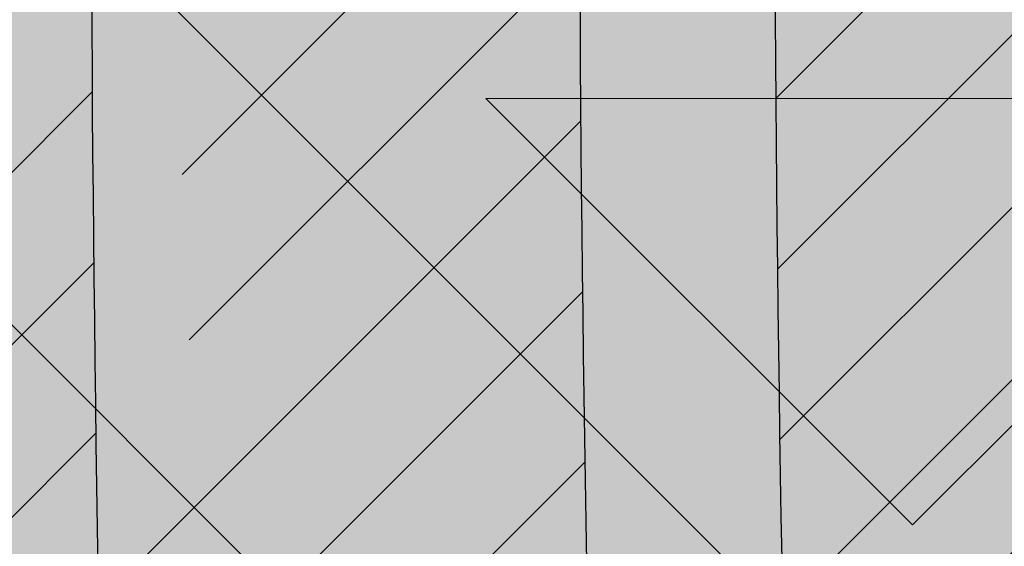
# Model space of a CAD drawing. Units: inches. Extents: x 844 to 2234, y 346 to 1084.
# Tile 11 of 93: x 1120.394 to 1122.002, y 692.842 to 693.702. Entities that reach past the tile are written whole.
import ezdxf

# ---------------------------------------------------------------- set-up
doc = ezdxf.new("R2010")
doc.units = ezdxf.units.IN
doc.header["$MEASUREMENT"] = 0
for name, color, linetype, lineweight in [('A-ANNO-DIMS', 2, 'Continuous', 18), ('furniture', 8, 'Continuous', 18), ('RA-AP-01$0$INT', 35, 'Continuous', 5)]:
    doc.layers.add(name, color=color, linetype=linetype, lineweight=lineweight)
doc.layers.add('RA-AP-01$0$FURN', color=3, linetype='Continuous')
doc.layers.add('RA-AP-01$0$WOOD', color=64, linetype='Continuous')
doc.styles.get("Standard").update_dxf_attribs({"font": 'arial.ttf'})
doc.dimstyles.get("Standard").update_dxf_attribs({"dimtxt": 6, "dimasz": 3, "dimexe": 0.18, "dimexo": 0.0625, "dimgap": 0.09, "dimtad": 0, "dimtih": 1, "dimtoh": 1, "dimdec": 1, "dimzin": 0, "dimdsep": 46, "dimlunit": 3, "dimtxsty": 'Standard', "dimblk": 'ARCHTICK', "dimcen": 0.09, "dimadec": 0, "dimazin": 0, "dimtfac": 1, "dimtdec": 1, "dimtofl": 0, "dimtmove": 0, "dimatfit": 3, "dimfxl": 1, "dimtolj": 1, "dimtzin": 0, "dimarcsym": 0})

# ---------------------------------------------------------------- blocks, each defined once
blk = doc.blocks.new('A$C18D01794')
at = {"layer": 'RA-AP-01$0$INT'}
h = blk.add_hatch(color=256, dxfattribs=at)
h.paths.add_polyline_path([(4.585917135068449, -6.356712009588271), (4.555206456959269, -6.35671200958746), (4.555206456959137, -6.387422687716308), (4.874495778835233, -6.706712009592356), (4.90520645695423, -6.676001331474049)])
h.paths.add_polyline_path([(5.255206456948813, -6.387422687716306), (5.255206456948682, -6.356712009605972), (5.224495778822613, -6.356712009605161), (4.905206456953498, -6.676001331474273), (4.935917135072151, -6.706712009592924)])
h.paths.add_polyline_path([(4.935917135072559, -6.706712009592068), (4.905206456953564, -6.737422687710376), (5.255206456951813, -7.087422687708613), (5.255206456951549, -7.026001331471008)])
h.paths.add_polyline_path([(4.555206456956399, -7.026001331471013), (4.555206456956134, -7.087422687708616), (4.905206456953821, -6.737422687710943), (4.874495778835166, -6.70671200959229)])
h = blk.add_hatch(color=256, dxfattribs=at)
h.paths.add_polyline_path([(4.585917135068448, -6.356712009588273), (4.614201406330596, -6.356712009589021), (4.668846067270487, -6.411356670531338), (4.723490728212344, -6.356712009591912), (4.771774999457151, -6.35671200959319), (4.826419660396886, -6.411356670535356), (4.862780050090322, -6.374996280843536), (4.844495778842715, -6.356712009595112), (4.862780050090411, -6.356712009595595), (4.905206456960182, -6.399138416468211), (4.947632863832445, -6.356712009597838), (4.965917135079675, -6.356712009598322), (4.947632863831759, -6.374996280845421), (4.983993253523576, -6.411356670538857), (5.038637914464627, -6.356712009600247), (5.08692218571208, -6.356712009601523), (5.141566846649976, -6.411356670541852), (5.196211507589851, -6.356712009604411), (5.224495778822615, -6.356712009605161), (4.905206456953975, -6.676001331473793)])
h.paths.add_polyline_path([(4.895206456956031, -6.637717060225675), (4.895206456958921, -6.528427738347902), (4.840561796018589, -6.583072399285802)], flags=16)
h.paths.add_polyline_path([(4.915206456955638, -6.637717060226121), (4.969851117895509, -6.583072399288678), (4.915206456957609, -6.528427738348344)], flags=16)
h.paths.add_polyline_path([(4.826419660395175, -6.568930263661755), (4.881064321335613, -6.514285602723745), (4.771774999456703, -6.514285602720857)], flags=16)
h.paths.add_polyline_path([(4.983993253519558, -6.568930263665262), (5.038637914460456, -6.514285602726792), (4.929348592581548, -6.514285602724816)], flags=16)
h.paths.add_polyline_path([(4.881064321336025, -6.494285602723742), (4.826419660397532, -6.439640941782821), (4.771774999457062, -6.494285602720859)], flags=16)
h.paths.add_polyline_path([(4.929348592582019, -6.494285602724817), (5.038637914460982, -6.494285602726792), (4.983993253522945, -6.439640941786327)], flags=16)
h.paths.add_polyline_path([(4.895206456960191, -6.480143467100443), (4.895206456962115, -6.407422687715913), (4.876922185715016, -6.389138416467584), (4.840561796021581, -6.425498806159401)], flags=16)
h.paths.add_polyline_path([(4.915206456958487, -6.480143467100889), (4.969851117899527, -6.425498806162279), (4.933490728206909, -6.389138416468043), (4.9152064569598, -6.40742268771434)], flags=16)
h.paths.add_polyline_path([(4.757632863832376, -6.480143467096812), (4.812277524772842, -6.425498806158772), (4.757632863834348, -6.370854145217844)], flags=16)
h.paths.add_polyline_path([(4.737632863832376, -6.480143467096286), (4.737632863834348, -6.370854145217375), (4.682988202893906, -6.425498806155385)], flags=16)
h.paths.add_polyline_path([(5.05278005008503, -6.480143467103376), (5.052780050087917, -6.370854145224413), (4.998135389146995, -6.425498806162908)], flags=16)
h.paths.add_polyline_path([(5.072780050085024, -6.480143467103744), (5.127424711025931, -6.42549880616527), (5.072780050087916, -6.370854145224832)], flags=16)
h.paths.add_polyline_path([(4.935917135072783, -6.706712009592292), (5.255206456948811, -6.387422687716309), (5.255206456948932, -6.415706958964177), (5.200561796010279, -6.470351619902839), (5.255206456949403, -6.524996280841948), (5.25520645694961, -6.5732805520894), (5.200561796009787, -6.627925213029239), (5.236922185702417, -6.664285602721864), (5.255206456949919, -6.646001331474357), (5.255206456949998, -6.664285602721898), (5.212780050078687, -6.706712009592262), (5.25520645695036, -6.749138416463932), (5.255206456950438, -6.767422687711313), (5.236922185702424, -6.749138416463297), (5.200561796009796, -6.785498806155928), (5.255206456950753, -6.840143467096874), (5.25520645695096, -6.888427738341682), (5.200561796010322, -6.943072399282328), (5.255206456951428, -6.997717060223427), (5.255206456951547, -7.026001331471006)])
h.paths.add_polyline_path([(5.042988202883395, -6.785498806155427), (5.097632863823085, -6.840143467095101), (5.097632863822622, -6.730854145216193)], flags=16)
h.paths.add_polyline_path([(5.028846067259663, -6.771356670531693), (5.083490728198774, -6.716712009592573), (4.974201406321001, -6.716712009593042)], flags=16)
h.paths.add_polyline_path([(5.117632863823087, -6.840143467095186), (5.172277524762331, -6.785498806155926), (5.11763286382262, -6.730854145216225)], flags=16)
h.paths.add_polyline_path([(5.08349072819877, -6.696712009593886), (5.028846067259652, -6.642067348654775), (4.974201406320998, -6.696712009593438)], flags=16)
h.paths.add_polyline_path([(5.131774999446817, -6.854285602718917), (5.186419660386065, -6.799640941779662), (5.241064321325782, -6.854285602719365)], flags=17)
h.paths.add_polyline_path([(5.131774999446228, -6.716712009592374), (5.186419660386065, -6.771356670532194), (5.222780050079488, -6.734996280838764), (5.204495778832781, -6.716712009592063)], flags=16)
h.paths.add_polyline_path([(5.097632863822613, -6.682569873970264), (5.097632863823061, -6.573280552091354), (5.042988202883383, -6.627925213031044)], flags=16)
h.paths.add_polyline_path([(5.131774999446899, -6.874285602718915), (5.241064321325809, -6.874285602719364), (5.186419660386591, -6.928930263658598)], flags=17)
h.paths.add_polyline_path([(5.131774999446226, -6.696712009594078), (5.204495778830767, -6.696712009594374), (5.22278005007868, -6.67842773834687), (5.186419660386049, -6.642067348654249)], flags=16)
h.paths.add_polyline_path([(5.11763286382262, -6.682569873970225), (5.17227752476232, -6.627925213030515), (5.117632863823064, -6.573280552091267)], flags=16)
h.paths.add_polyline_path([(5.186419660386069, -6.613783077405491), (5.241064321325754, -6.559138416465795), (5.131774999446791, -6.559138416466263)], flags=16)
h.paths.add_polyline_path([(5.131774999446872, -6.539138416466263), (5.24106432132578, -6.539138416465794), (5.186419660386554, -6.484493755526573)], flags=16)
h.paths.add_polyline_path([(5.255206456951811, -7.08742268770861), (5.255206456951895, -7.106712009588038), (4.555206456956052, -7.106712009588038), (4.555206456956136, -7.087422687708617), (4.905206456953973, -6.737422687710788)])
h.paths.add_polyline_path([(4.983993253513404, -6.8444937555241), (4.92934859257295, -6.899138416462108), (5.03863791445186, -6.899138416465014)], flags=16)
h.paths.add_polyline_path([(4.969851117889988, -6.83035161990006), (4.915206456952556, -6.775706958960171), (4.915206456949648, -6.884996280837944)], flags=16)
h.paths.add_polyline_path([(4.929348592572535, -6.919138416462105), (4.983993253511019, -6.973783077403037), (5.038637914451496, -6.919138416465012)], flags=16)
h.paths.add_polyline_path([(5.052780050074912, -6.93328055208906), (4.998135389134438, -6.987925213027088), (5.052780050072919, -7.042569873968025)], flags=16)
h.paths.add_polyline_path([(5.07278005007491, -6.933280552089588), (5.072780050072918, -7.042569873968497), (5.127424711013374, -6.987925213030498)], flags=16)
h.paths.add_polyline_path([(4.89520645695295, -6.775706958959721), (4.840561796013067, -6.830351619897157), (4.895206456950961, -6.884996280837494)], flags=16)
h.paths.add_polyline_path([(4.915206456948365, -6.933280552085403), (4.915206456946434, -7.006001331471951), (4.933490728192729, -7.024285602719066), (4.969851117886972, -6.987925213026453)], flags=16)
h.paths.add_polyline_path([(4.881064321327021, -6.899138416461022), (4.82641966038902, -6.84449375552057), (4.771774999448108, -6.899138416459029)], flags=16)
h.paths.add_polyline_path([(4.895206456950073, -6.933280552084951), (4.840561796009022, -6.987925213023558), (4.876922185700835, -7.024285602716997), (4.895206456948749, -7.006001331469487)], flags=16)
h.paths.add_polyline_path([(4.983993253510392, -7.0020673486505), (4.947632863816944, -7.038427738342319), (4.965917135064043, -7.05671200959023), (5.038637914448995, -7.056712009591555)], flags=16)
h.paths.add_polyline_path([(4.881064321326543, -6.91913841646102), (4.771774999447578, -6.919138416459031), (4.826419660385607, -6.973783077399508)], flags=16)
h.paths.add_polyline_path([(4.905206456946447, -7.014285602717636), (4.862780050074785, -7.056712009588352), (4.947632863816685, -7.056712009589775)], flags=16)
h.paths.add_polyline_path([(5.14156684663679, -7.002067348654549), (5.086922185696452, -7.056712009592438), (5.196211507574223, -7.056712009594425)], flags=16)
h.paths.add_polyline_path([(4.8264196603837, -7.002067348646972), (4.771774999442643, -7.056712009585575), (4.8444957788276, -7.056712009587508), (4.862780050075511, -7.038427738340416)], flags=16)
h.paths.add_polyline_path([(4.812277524760289, -6.98792521302292), (4.757632863822258, -6.933280552082447), (4.757632863819352, -7.042569873961408)], flags=16)
h.paths.add_polyline_path([(4.73763286382226, -6.933280552082079), (4.682988202881349, -6.987925213020536), (4.737632863819352, -7.04256987396099)], flags=16)
h.paths.add_polyline_path([(4.723490728195188, -7.056712009584289), (4.668846067257299, -7.002067348643949), (4.614201406317417, -7.056712009581383)], flags=16)
h.paths.add_polyline_path([(4.597632863829262, -6.706712009592262), (4.555206456957951, -6.664285602721896), (4.555206456958029, -6.646001331474357), (4.573490728205535, -6.664285602721864), (4.609851117898167, -6.627925213029238), (4.555206456958338, -6.573280552089402), (4.555206456958546, -6.524996280841952), (4.60985111789767, -6.470351619902839), (4.555206456959015, -6.415706958964177), (4.555206456959138, -6.387422687716309), (4.874495778835167, -6.70671200959229), (4.5552064569564, -7.026001331471015), (4.555206456956523, -6.997717060223433), (4.609851117897629, -6.94307239928233), (4.555206456956988, -6.888427738341681), (4.555206456957198, -6.840143467096881), (4.609851117898153, -6.78549880615593), (4.573490728205528, -6.749138416463297), (4.555206456957507, -6.76742268771132), (4.555206456957585, -6.749138416463933)])
h.paths.add_polyline_path([(4.712780050085332, -6.730854145216195), (4.712780050084863, -6.840143467095105), (4.767424711024555, -6.785498806155427)], flags=16)
h.paths.add_polyline_path([(4.726922185709173, -6.716712009592573), (4.781566846648288, -6.771356670531693), (4.836211507586949, -6.716712009593043)], flags=16)
h.paths.add_polyline_path([(4.692780050085327, -6.730854145216225), (4.638135389145619, -6.785498806155928), (4.692780050084865, -6.840143467095185)], flags=16)
h.paths.add_polyline_path([(4.726922185709182, -6.696712009593886), (4.836211507586949, -6.696712009593436), (4.7815668466483, -6.642067348654773)], flags=16)
h.paths.add_polyline_path([(4.678637914461726, -6.71671200959237), (4.605917135075169, -6.716712009592063), (4.587632863828464, -6.734996280838766), (4.623993253521887, -6.771356670532195)], flags=16)
h.paths.add_polyline_path([(4.712780050085336, -6.68256987397026), (4.767424711024568, -6.627925213031042), (4.71278005008489, -6.573280552091352)], flags=16)
h.paths.add_polyline_path([(4.678637914461726, -6.696712009594076), (4.623993253521899, -6.642067348654247), (4.587632863829271, -6.67842773834687), (4.605917135077185, -6.696712009594376)], flags=16)
h.paths.add_polyline_path([(4.692780050085336, -6.682569873970228), (4.692780050084889, -6.573280552091267), (4.638135389145632, -6.627925213030515)], flags=16)
h.paths.add_polyline_path([(4.623993253521885, -6.799640941779662), (4.678637914461131, -6.854285602718915), (4.56934859258217, -6.854285602719365)], flags=17)
h.paths.add_polyline_path([(4.623993253521901, -6.613783077405509), (4.678637914461158, -6.559138416466263), (4.569348592582195, -6.559138416465795)], flags=16)
h.paths.add_polyline_path([(4.678637914461051, -6.874285602718915), (4.623993253521361, -6.928930263658598), (4.569348592582143, -6.874285602719364)], flags=17)
h.paths.add_polyline_path([(4.678637914461076, -6.539138416466263), (4.623993253521399, -6.484493755526573), (4.569348592582167, -6.539138416465796)], flags=16)
h = blk.add_hatch(color=256, dxfattribs=at)
h.paths.add_polyline_path([(4.895206456952951, -6.77570695895972), (4.840561796013068, -6.830351619897156), (4.895206456950958, -6.884996280837495)])
h.paths.add_polyline_path([(4.915206456949649, -6.884996280837942), (4.969851117889987, -6.830351619900054), (4.915206456952556, -6.775706958960171)])
h.paths.add_polyline_path([(5.038637914451862, -6.899138416465013), (4.983993253513403, -6.8444937555241), (4.929348592572953, -6.899138416462106)])
h.paths.add_polyline_path([(4.929348592572535, -6.919138416462105), (4.983993253511018, -6.973783077403037), (5.038637914451497, -6.919138416465012)])
h.paths.add_polyline_path([(4.915206456948366, -6.933280552085397), (4.915206456946433, -7.006001331471951), (4.93349072819273, -7.024285602719068), (4.969851117886972, -6.987925213026454)])
h.paths.add_polyline_path([(5.038637914448995, -7.056712009591553), (4.983993253510389, -7.002067348650502), (4.947632863816946, -7.038427738342318), (4.965917135064043, -7.05671200959023)])
h.paths.add_polyline_path([(5.05278005007292, -7.042569873968023), (5.05278005007491, -6.933280552089059), (4.998135389134438, -6.987925213027088)])
h.paths.add_polyline_path([(5.07278005007292, -7.042569873968496), (5.127424711013374, -6.987925213030498), (5.072780050074909, -6.933280552089588)])
h.paths.add_polyline_path([(5.141566846636789, -7.002067348654547), (5.086922185696449, -7.056712009592438), (5.196211507574223, -7.056712009594425)])
h.paths.add_polyline_path([(4.947632863816688, -7.056712009589774), (4.905206456946449, -7.014285602717634), (4.862780050074784, -7.056712009588353)])
h.paths.add_polyline_path([(4.840561796009025, -6.987925213023556), (4.876922185700834, -7.024285602716997), (4.895206456948747, -7.006001331469488), (4.895206456950075, -6.933280552084953)])
h.paths.add_polyline_path([(4.88106432132654, -6.919138416461021), (4.771774999447577, -6.919138416459031), (4.826419660385606, -6.973783077399508)])
h.paths.add_polyline_path([(4.881064321327019, -6.899138416461022), (4.826419660389019, -6.844493755520571), (4.771774999448108, -6.89913841645903)])
h.paths.add_polyline_path([(4.757632863819352, -7.042569873961409), (4.812277524760284, -6.987925213022922), (4.757632863822259, -6.933280552082447)])
h.paths.add_polyline_path([(4.8264196603837, -7.002067348646974), (4.771774999442646, -7.056712009585575), (4.844495778827599, -7.05671200958751), (4.862780050075512, -7.038427738340417)])
h.paths.add_polyline_path([(4.737632863819352, -7.042569873960988), (4.737632863822258, -6.933280552082078), (4.682988202881349, -6.987925213020538)])
h.paths.add_polyline_path([(4.668846067257299, -7.002067348643952), (4.61420140631742, -7.056712009581384), (4.723490728195189, -7.056712009584292)])
for p, q in [((4.874495778835167, -6.70671200959229), (4.555206456956399, -7.026001331471013)), ((4.905206456953975, -6.737422687710788), (4.555206456956136, -7.087422687708617)), ((4.826419660389018, -6.844493755520574), (4.771774999448109, -6.899138416459031)), ((4.881064321327019, -6.899138416461022), (4.82641966038902, -6.844493755520572)), ((4.771774999448109, -6.899138416459031), (4.881064321327019, -6.899138416461022))]:
    blk.add_line(p, q, dxfattribs=at)
blk = doc.blocks.new('A$C32926AE1')
at = {"layer": 'RA-AP-01$0$FURN'}
h = blk.add_hatch(dxfattribs=at)
h.set_pattern_fill('ANSI31', color=256, scale=0.1, style=0)
h.set_pattern_definition([(45, (0, 0), (-0.0088388347648318, 0.0088388347648318), [])])
edge = h.paths.add_edge_path(flags=16)
edge.add_arc((4.904771284329206, 4.246793130718756), 0.2603971832811541, 75.22398030683196, 104.7760196931204)
edge.add_arc((4.904771284329206, 4.246793130718756), 0.2603971832811541, 75.223980306832, 104.77601969312039, ccw=False)
edge = h.paths.add_edge_path(flags=16)
edge.add_arc((4.904771284329206, 4.067062675376612), 0.2603971832811541, 255.2239803068796, 284.776019693168)
edge.add_arc((4.904771284329206, 4.067062675376612), 0.2603971832811541, 255.22398030687958, 284.77601969316805, ccw=False)
edge = h.paths.add_edge_path(flags=0)
edge.add_arc((4.904771284329206, 4.067062675376612), 0.2603971832811541, 255.2239803068796, 284.776019693168)
edge.add_arc((4.904771284329206, 4.067062675376612), 0.2603971832811541, 255.22398030687958, 284.77601969316805, ccw=False)
edge = h.paths.add_edge_path(flags=0)
edge.add_arc((4.904771284329206, 4.067062675376612), 0.2603971832811541, 255.2239803068796, 284.776019693168)
edge.add_arc((4.904771284329206, 4.067062675376612), 0.2603971832811541, 255.22398030687958, 284.77601969316805, ccw=False)
edge = h.paths.add_edge_path()
edge.add_arc((4.604388392048174, 4.588829985554312), 0.1599999999999918, 342.3781640246255, 354.4317409793762)
edge.add_arc((5.090145208887507, 4.43216705527679), 0.3503971832811637, 162.0091218307731, 180.3186872093483)
edge.add_arc((5.205154176610243, 4.588829985554953), 0.1599999999999917, 185.5682590208461, 197.6218359767349)
edge.add_arc((4.904771284329229, 4.246793130718735), 0.3503971832811761, 72.00912183053516, 107.9908781690354)
edge.add_arc((9.535952835716557, 4.28682295566602), 4.798342501046485, 178.2875002453811, 181.5576802719453)
edge.add_arc((4.719397359771122, 4.43216705527679), 0.3503971832811637, 359.6813127906516, 377.9908781692269)
edge.add_arc((9.535967292294904, 4.286822350292874), 4.778371420254705, 178.2965938931842, 181.5667745797229)
edge.add_arc((4.719397359771122, 4.43216705527679), 0.3303971832811637, 359.6813127906516, 377.9908781692269)
edge.add_arc((0.2735752763637294, 4.286822350292874), 4.7783714202547, 358.4332254202771, 361.7034061068158)
edge.add_arc((5.061434214606998, 4.732549947558029), 0.1600000000000254, 252.3781640250584, 264.4317409792362)
edge.add_arc((4.748108354051257, 4.732549947558012), 0.1600000000000541, 275.5682590208426, 287.6218359759532)
edge.add_arc((4.604388392048115, 4.588829985554317), 0.1800000000000505, 342.3567572500182, 349.3735009646207)
edge.add_arc((5.205154176610254, 4.588829985554976), 0.1800000000000069, 190.6264990356027, 197.6432427513933)
edge.add_arc((5.061434214607106, 4.732549947558013), 0.1800000000000424, 252.3567572496606, 259.3735009644582)
edge.add_arc((4.904771284329208, 4.246793130718737), 0.3303971832811676, 71.99844483668534, 108.0015551637021)
edge.add_arc((4.748108354051414, 4.732549947558045), 0.1800000000000547, 280.6264990355479, 287.6432427495938)
edge.add_arc((5.090145208887514, 4.432167055276789), 0.2803971832811691, 162.8706300666893, 180.816523289902)
edge.add_arc((4.719397359771136, 4.432167055276689), 0.2803971832811534, 359.183476710103, 377.1293699333214)
edge.add_arc((4.904771284329222, 4.246793130718737), 0.2803971832811769, 72.87063006672916, 107.1293699332334)
edge.add_arc((5.090145208887522, 4.432167055276788), 0.2603971832811776, 165.2239803068007, 180.9953123810312)
edge.add_arc((4.719397359771141, 4.432167055276699), 0.2603971832811458, 359.0046876189768, 374.7760196932087)
edge.add_arc((5.090145208887507, 4.43216705527679), 0.3303971832811637, 162.0091218307731, 180.3186872093483)
edge.add_arc((9.53595427642584, 4.285015535491528), 4.728345371032053, 178.265043920078, 181.5679956281801)
edge.add_arc((0.2735882922327999, 4.285015535491582), 4.728345371032045, 358.4320043718193, 361.7349560799204)
edge.add_arc((9.535953591267507, 4.284458026472751), 4.708343996644348, 178.2573054306777, 181.5704995759608)
edge.add_arc((0.273588977391114, 4.284458026472785), 4.708343996644358, 358.4295004240388, 361.7426945693213)
edge.add_arc((0.2735889773911131, 4.029397779622582), 4.708343996644359, 358.2573054306787, 361.5704995759613)
edge.add_arc((9.535953591267518, 4.029397779622618), 4.708343996644359, 178.4295004240391, 181.7426945693223)
edge.add_arc((0.2735882922327901, 4.028840270603786), 4.728345371032054, 358.2650439200796, 361.5679956281808)
edge.add_arc((9.53595427642584, 4.028840270603841), 4.728345371032054, 178.4320043718199, 181.7349560799219)
edge.add_arc((0.2735752763637302, 4.027033455802493), 4.778371420254699, 358.2965938931842, 361.5667745797229)
edge.add_arc((4.719397359771122, 3.881688750818578), 0.3303971832811637, 342.0091218307731, 360.3186872093484)
edge.add_arc((5.090145208887507, 3.881688750818578), 0.3303971832811637, 179.6813127906516, 197.9908781692269)
edge.add_arc((9.535967292294904, 4.027033455802493), 4.778371420254705, 178.433225420277, 181.7034061068158)
edge.add_arc((4.719397359771122, 3.881688750818578), 0.3503971832811637, 342.0091218307731, 360.3186872093484)
edge.add_arc((9.53595283571655, 4.027032850429349), 4.79834250104648, 178.4423197280546, 181.7124997546188)
edge.add_arc((4.719397359771141, 3.881688750818669), 0.2603971832811458, 345.2239803067913, 360.9953123810232)
edge.add_arc((5.090145208887522, 3.88168875081858), 0.2603971832811776, 179.0046876189687, 194.7760196931993)
edge.add_arc((4.904771284329222, 4.067062675376631), 0.2803971832811769, 252.8706300667665, 287.1293699332708)
edge.add_arc((4.719397359771136, 3.881688750818678), 0.2803971832811534, 342.8706300666787, 360.8165232898969)
edge.add_arc((5.090145208887514, 3.881688750818579), 0.2803971832811691, 179.183476710098, 197.1293699333106)
edge.add_arc((4.748108354051414, 3.581305858537323), 0.1800000000000547, 72.3567572504062, 79.37350096445199)
edge.add_arc((4.904771284329208, 4.067062675376631), 0.3303971832811676, 251.9984448362979, 288.0015551633146)
edge.add_arc((5.061434214607106, 3.581305858537355), 0.1800000000000424, 100.6264990355418, 107.6432427503394)
edge.add_arc((5.205154176610254, 3.725025820540392), 0.1800000000000069, 162.3567572486066, 169.3735009643972)
edge.add_arc((4.604388392048115, 3.725025820541051), 0.1800000000000505, 10.62649903537925, 17.64324274998182)
edge.add_arc((4.748108354051257, 3.581305858537356), 0.1600000000000541, 72.37816402404681, 84.43174097915735)
edge.add_arc((4.904771284329229, 4.067062675376632), 0.3503971832811761, 252.0091218309645, 287.9908781694648)
edge.add_arc((5.061434214606998, 3.581305858537339), 0.1600000000000254, 95.56825902076373, 107.6218359749416)
edge.add_arc((5.205154176610243, 3.725025820540414), 0.1599999999999917, 162.3781640232651, 174.4317409791539)
edge.add_arc((5.090145208887507, 3.881688750818578), 0.3503971832811637, 179.6813127906516, 197.9908781692269)
edge.add_arc((4.604388392048174, 3.725025820541056), 0.1599999999999918, 5.568259020623824, 17.62183597537444)
edge.add_arc((0.2735897329420762, 4.28682295566602), 4.798342501046482, 358.4423197280547, 361.7124997546188)
edge.add_arc((0.2735897329420691, 4.027032850429348), 4.798342501046489, 358.2875002453812, 361.5576802719453)
at = {"layer": 'RA-AP-01$0$WOOD'}
h = blk.add_hatch(color=256, dxfattribs=at)
h.dxf.hatch_style = 1
h.paths.add_polyline_path([(5.157430609644524, 4.573483066760929, -0.1009492694046607), (5.155401577623758, 4.593365984175333, -0.1842662638101597), (5.172249623284174, 4.638795604568598, 0.2056608120311276), (5.179560981299304, 4.661316324430096, 0.3614336704623542), (5.134352340494423, 4.706524965234944, 0.2056608120311297), (5.111831620632933, 4.699213607219793, -0.1842662638101113), (5.066402000239693, 4.682365561559342, -0.1055311479399994), (5.045656153913092, 4.68467289944697, 0.1567636581983829), (4.763886414745334, 4.684672899446966, -0.1055311479399895), (4.743140568418733, 4.68236556155934, -0.1842662638100833), (4.6977109480255, 4.69921360721979, 0.2056608120302612), (4.675190228164109, 4.706524965234949, 0.3614336704708441), (4.629981587358889, 4.66131632442871, 0.2056608120245944), (4.637292945374126, 4.638795604567974, -0.1842662638101024), (4.654140991034615, 4.59336598417475, -0.1009492694055169), (4.652111959013835, 4.573483066760181, 0.021410119221476), (4.629748025606143, 4.156712009541676, 0.0214101192214795), (4.652111959013809, 3.739940952323101, -0.1009492694059586), (4.654140991034615, 3.720058034908448, -0.1842662638100975), (4.637292945374126, 3.674628414515226, 0.2056608120245705), (4.629981587358889, 3.652107694654492, 0.3614336704708879), (4.675190228164113, 3.606899053848249, 0.2056608120302384), (4.697710948025501, 3.614210411863408, -0.1842662638100995), (4.743140568418738, 3.63105845752386, -0.1055311479402541), (4.763886414745388, 3.628751119636215, 0.1567636581983776), (5.045656153913137, 3.628751119636244, -0.1055311479397538), (5.066402000239692, 3.631058457523857, -0.1842662638101067), (5.111831620632931, 3.614210411863407, 0.2056608120310924), (5.134352340494417, 3.606899053848256, 0.3614336704624001), (5.179560981299307, 3.652107694653103, 0.2056608120311314), (5.172249623284175, 3.6746284145146, -0.1842662638101402), (5.155401577623758, 3.72005803490786, -0.1009492694051366), (5.15743060964455, 3.739940952322354, 0.0214101192215073), (5.179794543052287, 4.156712009541468, 0.0214101192215252)])
h.paths.add_polyline_path([(4.639748609479751, 4.156712009541513, 0.0213537860821624), (4.661970494867118, 3.741887061152232, -0.094075836301374), (4.664143710413708, 3.7196126951003, -0.1824818158568985), (4.644813765429836, 3.668037719127816, 0.2056608120245319), (4.639939526753007, 3.653023905887301, 0.3614336704710246), (4.676106439397173, 3.616856993242342, 0.2056608120302234), (4.691120252638095, 3.621731231919122, -0.1824818158602558), (4.742695228611606, 3.641061176902986, -0.1029891339458722), (4.766991894714349, 3.638256818950944, 0.156709409989566), (5.042550673941472, 3.638256818950105, -0.102989133958497), (5.066847340047078, 3.641061176902949, -0.1824818158594995), (5.118422316020358, 3.621731231919103, 0.2056608120311416), (5.133436129261316, 3.616856993242346, 0.3614336704621468), (5.169603041905217, 3.653023905886178, 0.2056608120310986), (5.164728803228477, 3.668037719127177, -0.1824818158565612), (5.145398858244737, 3.719612695099578, -0.0940758363009313), (5.147572073791232, 3.741887061151398, 0.0213537860822023), (5.169793959178681, 4.156712009541451, 0.0213537860822226), (5.147572073791203, 4.571536957931898, -0.0940758363005034), (5.145398858244737, 4.59381132398362, -0.1824818158565587), (5.164728803228476, 4.645386299956021, 0.2056608120311045), (5.169603041905216, 4.66040011319702, 0.3614336704621845), (5.133436129261313, 4.696567025840856, 0.2056608120310773), (5.118422316020359, 4.691692787164098, -0.182481815859508), (5.066847340047078, 4.67236284218025, -0.1029891339584606), (5.04255067394148, 4.675167200133092, 0.156709409989566), (4.766991894714357, 4.675167200132257, -0.1029891339458842), (4.742695228611611, 4.672362842180213, -0.1824818158602725), (4.691120252638095, 4.691692787164077, 0.2056608120302152), (4.676106439397174, 4.696567025840858, 0.3614336704710363), (4.639939526753005, 4.660400113195899, 0.2056608120245495), (4.644813765429837, 4.645386299955384, -0.1824818158568934), (4.664143710413708, 4.593811323982902, -0.0940758363009187), (4.661970494867149, 4.571536957931074, 0.021353786082177)], flags=16)
h.paths.add_polyline_path([(5.129794543052235, 4.432167055276933, -0.0141661062790638), (5.130152669293814, 4.156927903047693, -0.0141661062790647), (5.129794543052234, 3.881688750818433, -0.0785247771143638), (5.10979738006795, 3.755143611847103, 0.0945969212073497), (5.105408519571111, 3.717898134952927, 0.1043170707844957), (5.116074640131521, 3.670385395016088, 0.1043170707864965), (5.068561900193738, 3.681051515576561, 0.09459692119553), (5.031316423304057, 3.676662655080835, -0.1580239521427272), (4.778226145355827, 3.676662655080367, 0.0945969211986668), (4.740980668464973, 3.681051515576592, 0.1043170707882822), (4.693467928526415, 3.670385395015844, 0.1043170707867916), (4.704134049087309, 3.717898134953662, 0.0945969211972894), (4.69974518859162, 3.755143611844042, -0.0785247771163196), (4.679748025606343, 3.881688750818406, -0.0141661062790663), (4.679389899364763, 4.156927903047693, -0.0141661062790672), (4.679748025606343, 4.432167055276998, -0.0785247771163064), (4.699745188591625, 4.55871219425134, 0.094596921197333), (4.704134049087308, 4.595957671141738, 0.1043170707867205), (4.693467928526416, 4.643470411079523, 0.1043170707882628), (4.740980668464965, 4.632804290518776, 0.0945969211988114), (4.778226145355874, 4.637193151015016, -0.158023952142669), (5.031316423304015, 4.637193151014546, 0.0945969211956361), (5.068561900193736, 4.632804290518806, 0.1043170707864979), (5.11607464013152, 4.643470411079278, 0.1043170707844617), (5.105408519571112, 4.595957671142455, 0.0945969212074597), (5.109797380067959, 4.558712194248236, -0.0785247771143467)], flags=0)
h.paths.add_polyline_path([(5.119794532311105, 4.432259799204851, -0.0142000800617244), (5.120156169157484, 4.156927903047701, -0.0142000800617277), (5.119794532311105, 3.881596006890482, -0.0784894509520253), (5.100273383573699, 3.758192358677797, 0.0940138827242913), (5.095413455884425, 3.717477693979438, 0.0606271852308753), (5.099615656341024, 3.686844378806616, 0.0606271852322524), (5.068982341167493, 3.691046579263239, 0.0940138827010453), (5.028267676478798, 3.686186651576848, -0.1580706864508061), (4.781274892180912, 3.686186651576435, 0.0940138827026903), (4.740560227491556, 3.691046579263279, 0.0606271852339895), (4.709926912317155, 3.686844378806508, 0.0606271852329405), (4.714129112773991, 3.717477693980356, 0.094013882701304), (4.709269185087677, 3.758192358669163, -0.0784894509577193), (4.689748036347473, 3.881596006890469, -0.014200080061729), (4.689386399501094, 4.156927903047709, -0.0142000800617217), (4.689748036347473, 4.432259799204808, -0.078489450957724), (4.709269185087651, 4.555663447426125, 0.0940138827014585), (4.714129112773992, 4.596378112114996, 0.0606271852329731), (4.709926912317154, 4.62701142728886, 0.0606271852340196), (4.74056022749157, 4.622809226832087, 0.0940138827024997), (4.781274892180847, 4.627669154518912, -0.1580706864508359), (5.028267676478777, 4.627669154518526, 0.0940138827010946), (5.068982341167492, 4.622809226832129, 0.060627185232254), (5.099615656341024, 4.627011427288751, 0.0606271852308727), (5.095413455884425, 4.59637811211593, 0.0940138827241088), (5.100273383573675, 4.555663447417647, -0.0784894509520978)], flags=0)
h.paths.add_polyline_path([(5.06978912287499, 4.430218106756144, -0.014241683694547), (5.070173729147532, 4.156927903047672, -0.0142416836945458), (5.06978912287499, 3.883637699339223, -0.0800609523125196), (5.052662118612511, 3.773463122773442, 0.0526421978001116), (5.04590916754064, 3.740550867606997, 0.0526421977992423), (5.012996912374707, 3.73379791653534, -0.1583028414718258), (4.796545656286308, 3.73379791653451, 0.0526421978034211), (4.763633401117837, 3.740550867607021, 0.0526421978018622), (4.756880450045755, 3.773463122774558, -0.0800609523117106), (4.739753445783639, 3.883637699339268, -0.0142416836945435), (4.739368839511098, 4.156927903047671, -0.0142416836945477), (4.739753445783639, 4.430218106756155, -0.0800609523116345), (4.75688045004574, 4.540392683320762, 0.052642197801941), (4.763633401117837, 4.573304938488346, 0.0526421978035071), (4.796545656286361, 4.580057889560873, -0.1583028414717561), (5.012996912374669, 4.580057889560039, 0.0526421977993048), (5.04590916754064, 4.57330493848837, 0.0526421978002057), (5.052662118612529, 4.540392683321868, -0.080060952312477)], flags=0)
h.paths.add_polyline_path([(5.049789715110557, 4.43038092723357, -0.0143097550741839), (5.05018085590259, 4.156927903047715, -0.0143097550741854), (5.049789715110558, 3.883474878861827, -0.0800685599149176), (5.03362098255317, 3.779581877367999, 0.0306258898956367), (5.028241146483733, 3.758218888663947, 0.0306258898977031), (5.006878157778253, 3.75283905259408, -0.1583983521624096), (4.802664410878162, 3.752839052594731, 0.0306258898946014), (4.781301422174808, 3.758218888663924, 0.0306258898967912), (4.775921586105202, 3.779581877368794, -0.080068559914251), (4.759752853548071, 3.883474878861786, -0.0143097550741854), (4.759361712756037, 4.156927903047671, -0.0143097550741854), (4.759752853548071, 4.430380927233557, -0.0800685599142479), (4.775921586105193, 4.534273928726546, 0.0306258898968306), (4.781301422174808, 4.555636917431444, 0.0306258898945754), (4.802664410878143, 4.561016753500631, -0.1583983521624168), (5.006878157778244, 4.561016753501291, 0.0306258898977177), (5.028241146483733, 4.555636917431421, 0.0306258898958182), (5.03362098255321, 4.534273928727244, -0.080068559914796)], flags=0)
h.paths.add_polyline_path([(4.999766070382627, 4.428171244713864, -0.0143443147609634), (5.000198441819402, 4.156927903047689, -0.0143443147609612), (4.999766070382627, 3.885684561381556, -0.0784641635803329), (4.987356730658798, 3.799103304488872, -0.1506053783831347), (4.822185837999821, 3.79910330448882, -0.0784641635803318), (4.809776498276007, 3.885684561381509, -0.014344314760963), (4.809344126839227, 4.156927903047677, -0.0143443147609645), (4.809776498276007, 4.428171244713873, -0.0784641635803192), (4.822185837999822, 4.514752501606549, -0.1506053783831338), (4.987356730658798, 4.514752501606494, -0.078464163580285)], flags=0)
h.paths.add_polyline_path([(4.979755254238824, 4.42764379880488, -0.0143772539198268), (4.980205517789977, 4.156927903047693, -0.0143772539198275), (4.979755254238824, 3.886212007290489, -0.0689242507424422), (4.971183264704897, 3.815276770442801, -0.1296645318904179), (4.838359303953726, 3.815276770442746, -0.0689242507424186), (4.829787314419809, 3.886212007290419, -0.0143772539198292), (4.829337050868653, 4.156927903047653, -0.0143772539198325), (4.829787314419809, 4.427643798804946, -0.0689242507424211), (4.838359303953725, 4.498579035652621, -0.1296645318904187), (4.971183264704897, 4.498579035652565, -0.0689242507424401)], flags=0)
h = blk.add_hatch(color=256, dxfattribs=at)
h.dxf.hatch_style = 1
h.paths.add_polyline_path([(5.145398858244737, 4.59381132398362, -0.1824818158565616), (5.164728803228476, 4.645386299956021, 0.2056608120311045), (5.169603041905216, 4.66040011319702, 0.3614336704621845), (5.133436129261313, 4.696567025840856, 0.2056608120310773), (5.118422316020359, 4.691692787164098, -0.182481815859508), (5.066847340047078, 4.67236284218025, -0.1029891339584606), (5.04255067394148, 4.675167200133092, 0.156709409989566), (4.766991894714357, 4.675167200132257, -0.1029891339458842), (4.742695228611611, 4.672362842180213, -0.1824818158602725), (4.691120252638095, 4.691692787164077, 0.2056608120302152), (4.676106439397174, 4.696567025840858, 0.3614336704710363), (4.639939526753005, 4.660400113195899, 0.2056608120245495), (4.644813765429837, 4.645386299955384, -0.1824818158568934), (4.664143710413708, 4.593811323982902, -0.0940758363009187), (4.661970494867149, 4.571536957931074, 0.0213537860821772), (4.639748609479751, 4.156712009541507, 0.0213537860821625), (4.661970494867119, 3.741887061152226, -0.0940758363013071), (4.664143710413708, 3.719612695100309, -0.1824818158569294), (4.644813765429836, 3.668037719127816, 0.2056608120245319), (4.639939526753007, 3.653023905887301, 0.3614336704710246), (4.676106439397173, 3.616856993242342, 0.2056608120302234), (4.691120252638095, 3.621731231919122, -0.1824818158602558), (4.742695228611606, 3.641061176902986, -0.1029891339458722), (4.766991894714349, 3.638256818950944, 0.156709409989566), (5.042550673941472, 3.638256818950105, -0.102989133958497), (5.066847340047078, 3.641061176902949, -0.1824818158594995), (5.118422316020358, 3.621731231919103, 0.2056608120311416), (5.133436129261316, 3.616856993242346, 0.3614336704621468), (5.169603041905217, 3.653023905886178, 0.2056608120310986), (5.164728803228477, 3.668037719127177, -0.1824818158565612), (5.145398858244737, 3.719612695099578, -0.0940758363009313), (5.147572073791232, 3.741887061151398, 0.0213537860822023), (5.169793959178681, 4.156712009541451, 0.0213537860822226), (5.147572073791203, 4.571536957931898, -0.0940758363004996)])
h.paths.add_polyline_path([(5.109797380067958, 4.55871219424824, -0.0785247771143472), (5.129794543052234, 4.432167055276936, -0.0141661062790644), (5.130152669293814, 4.156927903047685, -0.014166106279066), (5.129794543052234, 3.881688750818401, -0.0785247771143517), (5.109797380067946, 3.755143611847092, 0.0945969212073132), (5.105408519571111, 3.717898134952929, 0.1043170707844995), (5.116074640131521, 3.670385395016088, 0.1043170707864965), (5.068561900193738, 3.681051515576561, 0.09459692119553), (5.031316423304057, 3.676662655080835, -0.1580239521427272), (4.778226145355827, 3.676662655080367, 0.0945969211986668), (4.740980668464973, 3.681051515576592, 0.1043170707882822), (4.693467928526415, 3.670385395015844, 0.1043170707867916), (4.704134049087309, 3.717898134953662, 0.0945969211972894), (4.69974518859162, 3.755143611844042, -0.0785247771163196), (4.679748025606343, 3.881688750818406, -0.0141661062790663), (4.679389899364763, 4.156927903047693, -0.0141661062790672), (4.679748025606343, 4.432167055276998, -0.0785247771163064), (4.699745188591625, 4.55871219425134, 0.094596921197333), (4.704134049087308, 4.595957671141738, 0.1043170707867205), (4.693467928526416, 4.643470411079523, 0.1043170707882628), (4.740980668464965, 4.632804290518776, 0.0945969211988114), (4.778226145355874, 4.637193151015016, -0.158023952142669), (5.031316423304015, 4.637193151014546, 0.0945969211956361), (5.068561900193736, 4.632804290518806, 0.1043170707864979), (5.11607464013152, 4.643470411079278, 0.1043170707844617), (5.105408519571112, 4.595957671142455, 0.0945969212074504)], flags=16)
h.paths.add_polyline_path([(5.100273383573655, 4.55566344741771, -0.0784894509521388), (5.119794532311105, 4.432259799204852, -0.0142000800617252), (5.120156169157484, 4.156927903047686, -0.014200080061726), (5.119794532311105, 3.881596006890502, -0.0784894509520446), (5.100273383573696, 3.758192358677786, 0.0940138827242721), (5.095413455884425, 3.717477693979436, 0.0606271852308692), (5.099615656341024, 3.686844378806616, 0.0606271852322522), (5.068982341167493, 3.691046579263239, 0.0940138827010453), (5.028267676478798, 3.686186651576848, -0.1580706864508061), (4.781274892180912, 3.686186651576435, 0.0940138827026903), (4.740560227491556, 3.691046579263279, 0.0606271852339895), (4.709926912317155, 3.686844378806508, 0.0606271852329405), (4.714129112773991, 3.717477693980356, 0.094013882701304), (4.709269185087677, 3.758192358669163, -0.0784894509577193), (4.689748036347473, 3.881596006890469, -0.014200080061729), (4.689386399501094, 4.156927903047709, -0.0142000800617217), (4.689748036347473, 4.432259799204808, -0.078489450957724), (4.709269185087651, 4.555663447426125, 0.0940138827014585), (4.714129112773992, 4.596378112114996, 0.0606271852329731), (4.709926912317154, 4.62701142728886, 0.0606271852340196), (4.74056022749157, 4.622809226832087, 0.0940138827024997), (4.781274892180847, 4.627669154518912, -0.1580706864508359), (5.028267676478777, 4.627669154518526, 0.0940138827010946), (5.068982341167492, 4.622809226832129, 0.060627185232254), (5.099615656341024, 4.627011427288751, 0.0606271852308727), (5.095413455884425, 4.59637811211593, 0.094013882723957)], flags=0)
h.paths.add_polyline_path([(5.04590916754064, 4.57330493848837, 0.0526421978002057), (5.052662118612529, 4.540392683321868, -0.0800609523124783), (5.06978912287499, 4.430218106756142, -0.0142416836945469), (5.070173729147532, 4.156927903047672, -0.0142416836945458), (5.06978912287499, 3.883637699339223, -0.0800609523125196), (5.052662118612511, 3.773463122773442, 0.0526421978001116), (5.04590916754064, 3.740550867606997, 0.0526421977992423), (5.012996912374707, 3.73379791653534, -0.1583028414718258), (4.796545656286308, 3.73379791653451, 0.0526421978034211), (4.763633401117837, 3.740550867607021, 0.0526421978018622), (4.756880450045755, 3.773463122774558, -0.0800609523117106), (4.739753445783639, 3.883637699339268, -0.0142416836945435), (4.739368839511098, 4.156927903047671, -0.0142416836945477), (4.739753445783639, 4.430218106756155, -0.0800609523116345), (4.75688045004574, 4.540392683320762, 0.052642197801941), (4.763633401117837, 4.573304938488346, 0.0526421978035071), (4.796545656286361, 4.580057889560873, -0.1583028414717561), (5.012996912374669, 4.580057889560039, 0.0526421977993048)], flags=0)
h.paths.add_polyline_path([(5.028241146483733, 4.555636917431422, 0.0306258898956949), (5.033620982553182, 4.534273928727329, -0.0800685599148649), (5.049789715110557, 4.430380927233569, -0.0143097550741839), (5.05018085590259, 4.156927903047715, -0.0143097550741854), (5.049789715110558, 3.883474878861827, -0.0800685599149176), (5.03362098255317, 3.779581877367999, 0.0306258898956367), (5.028241146483733, 3.758218888663947, 0.0306258898977031), (5.006878157778253, 3.75283905259408, -0.1583983521624096), (4.802664410878162, 3.752839052594731, 0.0306258898946014), (4.781301422174808, 3.758218888663924, 0.0306258898967912), (4.775921586105202, 3.779581877368794, -0.080068559914251), (4.759752853548071, 3.883474878861786, -0.0143097550741854), (4.759361712756037, 4.156927903047671, -0.0143097550741854), (4.759752853548071, 4.430380927233557, -0.0800685599142479), (4.775921586105193, 4.534273928726546, 0.0306258898968306), (4.781301422174808, 4.555636917431444, 0.0306258898945754), (4.802664410878143, 4.561016753500631, -0.1583983521624168), (5.006878157778244, 4.561016753501291, 0.0306258898977174)], flags=0)
h.paths.add_polyline_path([(4.987356730658798, 4.514752501606494, -0.0784641635803018), (4.999766070382627, 4.428171244713845, -0.0143443147609637), (5.000198441819402, 4.156927903047665, -0.0143443147609622), (4.999766070382628, 3.885684561381514, -0.0784641635802952), (4.987356730658797, 3.799103304488872, -0.1506053783831338), (4.822185837999821, 3.799103304488819, -0.0784641635803342), (4.809776498276007, 3.885684561381512, -0.0143443147609628), (4.809344126839227, 4.156927903047676, -0.0143443147609646), (4.809776498276007, 4.428171244713873, -0.0784641635803192), (4.822185837999822, 4.514752501606549, -0.1506053783831338)], flags=0)
h.paths.add_polyline_path([(4.971183264704897, 4.498579035652566, -0.0689242507424384), (4.979755254238824, 4.427643798804883, -0.0143772539198276), (4.980205517789977, 4.15692790304768, -0.0143772539198258), (4.979755254238823, 3.88621200729051, -0.0689242507424628), (4.971183264704897, 3.815276770442801, -0.129664531890417), (4.838359303953726, 3.815276770442746, -0.0689242507424186), (4.829787314419809, 3.886212007290419, -0.0143772539198292), (4.829337050868653, 4.156927903047653, -0.0143772539198325), (4.829787314419809, 4.427643798804946, -0.0689242507424211), (4.838359303953725, 4.498579035652621, -0.1296645318904187)], flags=0)
h = blk.add_hatch(dxfattribs=at)
h.set_pattern_fill('ANSI31', color=256, scale=0.05, style=0)
h.set_pattern_definition([(45, (0, 0), (-0.0044194173824159, 0.0044194173824159), [])])
h.paths.add_polyline_path([(5.130152669293814, 4.156927903047704, 0.0141661062790657), (5.129794543052234, 4.432167055276982, 0.0777827904001433), (5.110168979996553, 4.557559993161921, -0.0976515123401879), (5.105408519571111, 4.595957671142454, -0.1043170707844687), (5.116074640131522, 4.64347041107928), (5.099615656341024, 4.627011427288751, 0.0606271852308727), (5.095413455884425, 4.59637811211593, 0.0940138827241088), (5.100273383573675, 4.555663447417647, -0.0784894509520972), (5.119794532311105, 4.432259799204852, -0.0142000800617252), (5.120156169157484, 4.156927903047686, -0.014200080061726), (5.119794532311105, 3.881596006890502, -0.0784894509520446), (5.100273383573696, 3.758192358677786, 0.0940138827242721), (5.095413455884425, 3.717477693979436, 0.0606271852308692), (5.099615656341024, 3.686844378806616), (5.116074640131519, 3.67038539501609, -0.1043170707844594), (5.105408519571112, 3.717898134952912, -0.0976515123401594), (5.11016897999655, 3.756295812933435, 0.0777827904001654), (5.129794543052234, 3.881688750818409, 0.0141661062790665)])
h.paths.add_polyline_path([(5.030164222210597, 3.676291055149937, -0.0976515123472002), (5.068561900193739, 3.681051515576561, -0.1043170707864927), (5.116074640131521, 3.670385395016088), (5.099615656341024, 3.686844378806616, 0.0606271852322522), (5.068982341167493, 3.691046579263239, 0.0940138827010453), (5.028267676478798, 3.686186651576848, -0.1580706864508061), (4.781274892180912, 3.686186651576435, 0.0940138827026903), (4.740560227491556, 3.691046579263279, 0.0606271852339913), (4.709926912317154, 3.686844378806508), (4.693467928526416, 3.670385395015845, -0.1043170707882796), (4.740980668464973, 3.681051515576592, -0.0976515123427246), (4.779378346446416, 3.676291055150394, 0.156512506893803)])
h.paths.add_polyline_path([(4.689748036347473, 3.881596006890472, -0.014200080061729), (4.689386399501094, 4.156927903047712, -0.0142000800617195), (4.689748036347473, 4.432259799204768, -0.078489450957742), (4.709269185087648, 4.555663447426114, 0.0940138827014821), (4.714129112773992, 4.596378112114995, 0.0606271852329748), (4.709926912317154, 4.62701142728886), (4.693467928526414, 4.643470411079524, -0.1043170707867939), (4.704134049087309, 4.595957671141706, -0.09765151234893), (4.699373588660725, 4.557559993157876, 0.0777827903975372), (4.679748025606343, 4.432167055276987, 0.0141661062790675), (4.679389899364763, 4.156927903047675, 0.0141661062790641), (4.679748025606343, 3.88168875081843, 0.0777827903975637), (4.699373588660724, 3.756295812937497, -0.0976515123490278), (4.704134049087308, 3.717898134953629, -0.1043170707867196), (4.693467928526416, 3.670385395015845), (4.709926912317155, 3.686844378806508, 0.0606271852329413), (4.714129112773991, 3.717477693980357, 0.0940138827013084), (4.709269185087676, 3.758192358669166, -0.0784894509577192)])
h.paths.add_polyline_path([(4.779378346446434, 4.63756475094498, -0.0976515123427943), (4.740980668464964, 4.632804290518776, -0.1043170707882609), (4.693467928526416, 4.643470411079523), (4.709926912317154, 4.62701142728886, 0.0606271852340196), (4.74056022749157, 4.622809226832087, 0.0940138827024997), (4.781274892180847, 4.627669154518912, -0.1580706864508359), (5.028267676478777, 4.627669154518526, 0.0940138827010946), (5.068982341167492, 4.622809226832129, 0.060627185232254), (5.099615656341024, 4.627011427288751), (5.116074640131521, 4.643470411079279, -0.1043170707865022), (5.068561900193735, 4.632804290518806, -0.0976515123475899), (5.030164222210446, 4.637564750945479, 0.1565125068936924)])
h = blk.add_hatch(dxfattribs=at)
h.set_pattern_fill('ANSI32', color=256, scale=0.2, style=0)
h.set_pattern_definition([(45, (0, 0), (-0.0530330085889911, 0.0530330085889911), []), (45, (0.035355339, 0), (-0.0530330085889911, 0.0530330085889911), [])])
h.paths.add_polyline_path([(5.119794532311105, 4.432259799204823, 0.0777015974868765), (5.10065834347252, 4.554469821747928, -0.0968902511992216), (5.095413455884425, 4.596378112115931, -0.060627185230871), (5.099615656341024, 4.627011427288751, -0.060627185232254), (5.068982341167492, 4.622809226832129, -0.0968902512198245), (5.027074050790956, 4.628054114423209, 0.1564657949319105), (4.782468517866163, 4.628054114422785, -0.0968902512152247), (4.740560227491555, 4.622809226832088, -0.0606271852339878), (4.709926912317155, 4.627011427288859, -0.0606271852329413), (4.714129112773991, 4.596378112115011, -0.0968902512205338), (4.708884225182929, 4.554469821738175, 0.0777015974804443), (4.689748036347473, 4.43225979920482, 0.0142000800617215), (4.689386399501094, 4.156927903047726, 0.0142000800617273), (4.689748036347473, 3.88159600689052, 0.077701597480541), (4.708884225182985, 3.759385984357019, -0.096890251220082), (4.714129112773992, 3.717477693980371, -0.0606271852329731), (4.709926912317154, 3.686844378806507, -0.060627185233988), (4.740560227491554, 3.691046579263279, -0.0968902512152569), (4.782468517866175, 3.685801691672578, 0.1564657949319236), (5.027074050790988, 3.685801691672169, -0.0968902512197451), (5.068982341167491, 3.691046579263239, -0.0606271852322557), (5.099615656341024, 3.686844378806616, -0.0606271852308727), (5.095413455884425, 3.717477693979438, -0.0968902511991229), (5.100658343472507, 3.7593859843474, 0.0777015974868745), (5.119794532311105, 3.8815960068905, 0.014200080061726), (5.120156169157484, 4.156927903047685, 0.0142000800617238)])
h.paths.add_polyline_path([(5.070173729147531, 4.156927903047684, -0.0142416836945481), (5.06978912287499, 3.883637699339191, -0.0800609523125107), (5.052662118612505, 3.773463122773424, 0.0526421978000811), (5.04590916754064, 3.740550867606997, 0.0526421977993214), (5.012996912374658, 3.733797916535325, -0.1583028414717916), (4.796545656286304, 3.733797916534512, 0.0526421978034138), (4.763633401117837, 3.740550867607021, 0.0526421978018622), (4.756880450045755, 3.773463122774558, -0.0800609523117106), (4.739753445783639, 3.883637699339268, -0.0142416836945435), (4.739368839511098, 4.156927903047671, -0.0142416836945477), (4.739753445783639, 4.430218106756155, -0.0800609523116345), (4.75688045004574, 4.540392683320762, 0.052642197801941), (4.763633401117837, 4.573304938488346, 0.0526421978035071), (4.796545656286361, 4.580057889560873, -0.1583028414717561), (5.012996912374669, 4.580057889560039, 0.0526421977993048), (5.04590916754064, 4.57330493848837, 0.0526421978002057), (5.052662118612529, 4.540392683321868, -0.0800609523124783), (5.06978912287499, 4.430218106756142, -0.0142416836945463)], flags=16)
h.paths.add_polyline_path([(5.050180855902591, 4.156927903047686, -0.0143097550741856), (5.049789715110558, 3.883474878861795, -0.0800685599148126), (5.033620982553202, 3.7795818773681, 0.0306258898957837), (5.028241146483733, 3.758218888663947, 0.0306258898977031), (5.006878157778253, 3.75283905259408, -0.1583983521624096), (4.802664410878162, 3.752839052594731, 0.0306258898946014), (4.781301422174808, 3.758218888663924, 0.0306258898967912), (4.775921586105202, 3.779581877368794, -0.080068559914251), (4.759752853548071, 3.883474878861786, -0.0143097550741854), (4.759361712756037, 4.156927903047671, -0.0143097550741854), (4.759752853548071, 4.430380927233557, -0.0800685599142479), (4.775921586105193, 4.534273928726546, 0.0306258898968306), (4.781301422174808, 4.555636917431444, 0.0306258898945754), (4.802664410878143, 4.561016753500631, -0.1583983521624168), (5.006878157778244, 4.561016753501291, 0.0306258898977177), (5.028241146483733, 4.555636917431421, 0.0306258898958182), (5.03362098255321, 4.534273928727244, -0.0800685599147973), (5.049789715110557, 4.430380927233568, -0.0143097550741854)], flags=0)
h.paths.add_polyline_path([(5.000198441819402, 4.15692790304769, -0.0143443147609622), (4.999766070382627, 3.885684561381539, -0.0784641635803169), (4.987356730658798, 3.799103304488873, -0.1506053783831347), (4.822185837999821, 3.79910330448882, -0.0784641635803318), (4.809776498276007, 3.885684561381509, -0.014344314760963), (4.809344126839227, 4.156927903047677, -0.0143443147609645), (4.809776498276007, 4.428171244713873, -0.0784641635803192), (4.822185837999822, 4.514752501606549, -0.1506053783831338), (4.987356730658798, 4.514752501606494, -0.0784641635803018), (4.999766070382627, 4.428171244713845, -0.0143443147609624)], flags=0)
h.paths.add_polyline_path([(4.980205517789976, 4.156927903047707, -0.0143772539198295), (4.979755254238824, 3.886212007290466, -0.06892425074242), (4.971183264704897, 3.815276770442801, -0.129664531890417), (4.838359303953726, 3.815276770442746, -0.0689242507424186), (4.829787314419809, 3.886212007290419, -0.0143772539198292), (4.829337050868653, 4.156927903047653, -0.0143772539198325), (4.829787314419809, 4.427643798804946, -0.0689242507424211), (4.838359303953725, 4.498579035652621, -0.1296645318904187), (4.971183264704897, 4.498579035652565, -0.0689242507424418), (4.979755254238824, 4.427643798804878, -0.0143772539198259)], flags=0)
for centre, radius, start, end in [((9.53595427642584, 4.028840270603841), 4.728345371032054, 178.4320043718199, 181.7349560799219), ((9.535953591267518, 4.029397779622618), 4.708343996644359, 178.4295004240391, 181.7426945693223), ((9.535967292294904, 4.027033455802493), 4.778371420254705, 178.433225420277, 181.7034061068158)]:
    blk.add_arc(centre, radius, start, end, dxfattribs=at)
blk = doc.blocks.new('A$C5D2F253E')
at = {"layer": 'RA-AP-01$0$FURN', "xscale": -0.7999999999883585, "yscale": 0.7999999999883585, "zscale": 0.8, "rotation": 90}
blk.add_blockref('A$C18D01794', (-5.687757199772477, 4.75791982714071), dxfattribs=at)
at = {"layer": 'RA-AP-01$0$WOOD', "rotation": 270}
blk.add_blockref('A$C32926AE1', (-4.161339601644158, 5.73852594588169), dxfattribs=at)
blk = doc.blocks.new('_ArchTick')
at = {"color": 0, "linetype": 'ByBlock', "const_width": 0.15}
blk.add_lwpolyline([(-0.5, -0.5), (0.5, 0.5)], dxfattribs=at)
blk = doc.blocks.new('*D144')
at = {"layer": 'A-ANNO-DIMS', "color": 0, "lineweight": -2, "transparency": 16777216}
for p, q in [((1096.615948, 439.3732739999999), (1096.615948, 1074.743301)), ((1143.115948, 492.373274), (1143.115948, 1074.743301)), ((1096.615948, 1074.563301), (1102.481950728513, 1074.563301)), ((1143.115948, 1074.563301), (1137.249945271487, 1074.563301))]:
    blk.add_line(p, q, dxfattribs=at)
at = {"layer": 'Defpoints', "color": 0, "transparency": 16777216}
for p in [(1143.115948, 1074.563301), (1143.115948, 492.3107739999999), (1096.615948, 439.3107739999999)]:
    blk.add_point(p, dxfattribs=at)
at = {"layer": 'A-ANNO-DIMS', "color": 0, "lineweight": -2, "transparency": 16777216, "xscale": 3, "yscale": 3, "zscale": 3, "rotation": 180}
blk.add_blockref('_ArchTick', (1096.615948, 1074.563301), dxfattribs=at)
at = {"layer": 'A-ANNO-DIMS', "color": 0, "lineweight": -2, "transparency": 16777216, "xscale": 3, "yscale": 3, "zscale": 3}
blk.add_blockref('_ArchTick', (1143.115948, 1074.563301), dxfattribs=at)
at = {"layer": 'A-ANNO-DIMS', "color": 0, "transparency": 16777216, "insert": (1119.865948, 1074.563301), "char_height": 6, "attachment_point": 5}
blk.add_mtext('\\A1;3\'-10 1/2"', dxfattribs=at)

msp = doc.modelspace()

# ---------------------------------------------------------------- block references
at = {"layer": 'furniture', "xscale": 15.94108302203742, "yscale": 15.94108302203742, "zscale": 15.94108302203742, "rotation": 90}
msp.add_blockref('A$C5D2F253E', (1136.147844094663, 696.2584716700112), dxfattribs=at)

# ---------------------------------------------------------------- dimensions: what is measured, and where the dimension line sits
at = {"layer": 'A-ANNO-DIMS'}
dim = msp.add_linear_dim(base=(1143.115948, 1074.563301), p1=(1096.615948, 439.3107739999999), p2=(1143.115948, 492.3107739999999), dimstyle='Standard', override={"dimdec": 1, "dimlfac": 1, "dimrnd": 0, "dimzin": 1, "dimdsep": 46, "dimlunit": 4, "dimfrac": 2}, dxfattribs=at)
dim.commit()
dim.dimension.update_dxf_attribs({"geometry": '*D144', "text_midpoint": (1119.865948, 1074.563301)})

doc.saveas('drawing.dxf')
